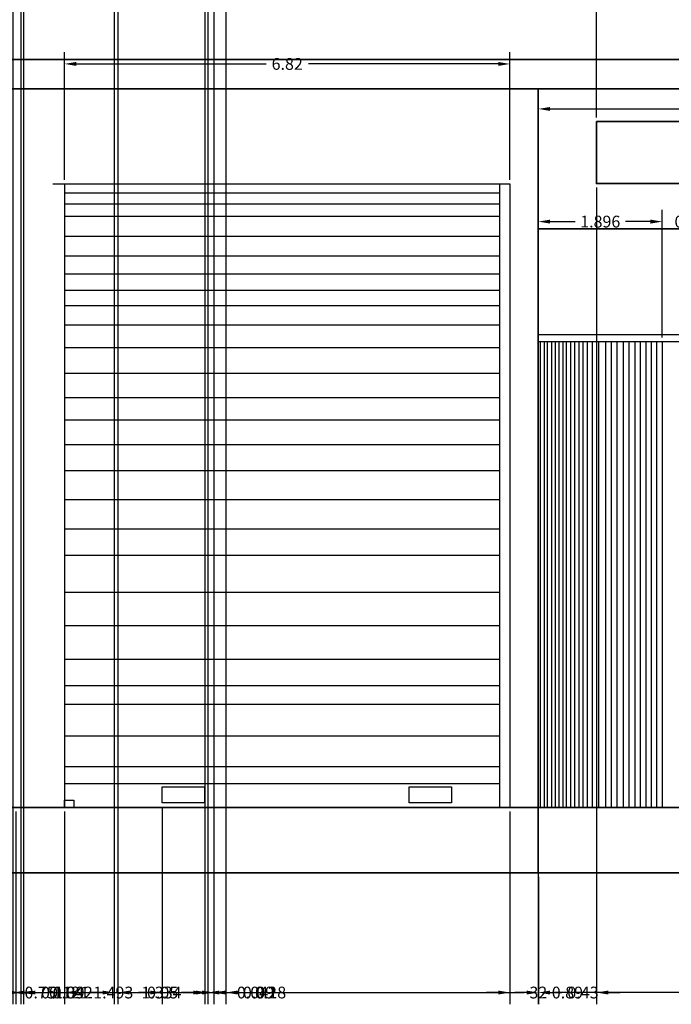
# Model space of a CAD drawing. Units: millimetres. Extents: x 2473 to 2512.3, y 2191.3 to 2230.4.
# Tile 2 of 8: x 2483.7 to 2493.7, y 2191.3 to 2206.4. Entities that reach past the tile are written whole.
import ezdxf

# ---------------------------------------------------------------- set-up
doc = ezdxf.new("R2010")
doc.units = ezdxf.units.MM
for name, color, linetype, lineweight in [('A-ANNO-DIMS', 2, 'Continuous', 18), ('A-DOOR', 4, 'Continuous', 25), ('A-ELEV', 7, 'Continuous', 35)]:
    doc.layers.add(name, color=color, linetype=linetype, lineweight=lineweight)
doc.styles.get("Standard").update_dxf_attribs({"font": 'arial.ttf'})
doc.dimstyles.get("Standard").update_dxf_attribs({"dimtxt": 0.18, "dimasz": 0.18, "dimexe": 0.18, "dimexo": 0.0625, "dimgap": 0.09, "dimtad": 0, "dimtih": 1, "dimtoh": 1, "dimdec": 4, "dimzin": 0, "dimdsep": 46, "dimtxsty": 'Standard', "dimcen": 0.09, "dimadec": 0, "dimazin": 0, "dimtfac": 1, "dimtdec": 4, "dimtofl": 0, "dimtmove": 0, "dimatfit": 3, "dimfxl": 1, "dimtolj": 1, "dimtzin": 0, "dimarcsym": 0})

# ---------------------------------------------------------------- blocks, each defined once
blk = doc.blocks.new('*D7')
at = {"layer": 'A-ANNO-DIMS', "color": 0, "lineweight": -2, "transparency": 16777216}
for p, q in [((2475.623, 2193.292), (2475.623, 2191.34)), ((2507.623, 2193.292), (2507.623, 2191.34)), ((2475.803, 2191.52), (2491.405, 2191.52)), ((2507.443, 2191.52), (2491.841, 2191.52))]:
    blk.add_line(p, q, dxfattribs=at)
at = {"layer": 'A-ANNO-DIMS', "color": 0, "transparency": 16777216}
for points in [[(2475.803, 2191.55), (2475.803, 2191.49), (2475.623, 2191.52)], [(2507.443, 2191.55), (2507.443, 2191.49), (2507.623, 2191.52)]]:
    blk.add_solid(points, dxfattribs=at)
at = {"layer": 'Defpoints', "color": 0, "transparency": 16777216}
for p in [(2475.623, 2193.355), (2507.623, 2193.355), (2507.623, 2191.52)]:
    blk.add_point(p, dxfattribs=at)
at = {"layer": 'A-ANNO-DIMS', "color": 0, "transparency": 16777216, "insert": (2491.623, 2191.52), "char_height": 0.18, "attachment_point": 5}
blk.add_mtext('\\A1;32', dxfattribs=at)
blk = doc.blocks.new('*D15')
at = {"layer": 'A-ANNO-DIMS', "color": 0, "lineweight": -2, "transparency": 16777216}
for p, q in [((2484.37, 2203.965), (2484.37, 2205.918)), ((2491.189, 2203.965), (2491.189, 2205.918)), ((2484.55, 2205.738), (2487.456, 2205.738)), ((2491.009, 2205.738), (2488.103, 2205.738))]:
    blk.add_line(p, q, dxfattribs=at)
at = {"layer": 'A-ANNO-DIMS', "color": 0, "transparency": 16777216}
for points in [[(2484.55, 2205.768), (2484.55, 2205.708), (2484.37, 2205.738)], [(2491.009, 2205.768), (2491.009, 2205.708), (2491.189, 2205.738)]]:
    blk.add_solid(points, dxfattribs=at)
at = {"layer": 'Defpoints', "color": 0, "transparency": 16777216}
for p in [(2491.189, 2205.738), (2484.37, 2203.903), (2491.189, 2203.903)]:
    blk.add_point(p, dxfattribs=at)
at = {"layer": 'A-ANNO-DIMS', "color": 0, "transparency": 16777216, "insert": (2487.779, 2205.738), "char_height": 0.18, "attachment_point": 5}
blk.add_mtext('\\A1;6.82', dxfattribs=at)
blk = doc.blocks.new('*D16')
at = {"layer": 'A-ANNO-DIMS', "color": 0, "lineweight": -2, "transparency": 16777216}
for p, q in [((2491.623, 2203.276), (2491.623, 2205.229)), ((2500.567, 2203.276), (2500.567, 2205.229)), ((2491.803, 2205.049), (2495.701, 2205.049)), ((2500.387, 2205.049), (2496.488, 2205.049))]:
    blk.add_line(p, q, dxfattribs=at)
at = {"layer": 'A-ANNO-DIMS', "color": 0, "transparency": 16777216}
for points in [[(2491.803, 2205.079), (2491.803, 2205.019), (2491.623, 2205.049)], [(2500.387, 2205.079), (2500.387, 2205.019), (2500.567, 2205.049)]]:
    blk.add_solid(points, dxfattribs=at)
at = {"layer": 'Defpoints', "color": 0, "transparency": 16777216}
for p in [(2500.567, 2205.049), (2491.623, 2203.214), (2500.567, 2203.214)]:
    blk.add_point(p, dxfattribs=at)
at = {"layer": 'A-ANNO-DIMS', "color": 0, "transparency": 16777216, "insert": (2496.095, 2205.049), "char_height": 0.18, "attachment_point": 5}
blk.add_mtext('\\A1;8.944', dxfattribs=at)
blk = doc.blocks.new('*D24')
at = {"layer": 'A-ANNO-DIMS', "color": 0, "lineweight": -2, "transparency": 16777216}
for p, q in [((2483.623, 2194.292), (2483.623, 2191.34)), ((2484.37, 2194.292), (2484.37, 2191.34)), ((2483.443, 2191.52), (2483.263, 2191.52)), ((2484.55, 2191.52), (2484.73, 2191.52))]:
    blk.add_line(p, q, dxfattribs=at)
at = {"layer": 'A-ANNO-DIMS', "color": 0, "transparency": 16777216}
for points in [[(2483.443, 2191.55), (2483.443, 2191.49), (2483.623, 2191.52)], [(2484.55, 2191.55), (2484.55, 2191.49), (2484.37, 2191.52)]]:
    blk.add_solid(points, dxfattribs=at)
at = {"layer": 'Defpoints', "color": 0, "transparency": 16777216}
for p in [(2483.623, 2194.355), (2484.37, 2194.355), (2484.37, 2191.52)]:
    blk.add_point(p, dxfattribs=at)
at = {"layer": 'A-ANNO-DIMS', "color": 0, "transparency": 16777216, "insert": (2483.996, 2191.52), "char_height": 0.18, "attachment_point": 5}
blk.add_mtext('\\A1;0.75', dxfattribs=at)
blk = doc.blocks.new('*D25')
at = {"layer": 'A-ANNO-DIMS', "color": 0, "lineweight": -2, "transparency": 16777216}
for p, q in [((2491.189, 2194.292), (2491.189, 2191.34)), ((2491.623, 2193.292), (2491.623, 2191.34)), ((2491.009, 2191.52), (2490.829, 2191.52)), ((2491.803, 2191.52), (2491.983, 2191.52))]:
    blk.add_line(p, q, dxfattribs=at)
at = {"layer": 'A-ANNO-DIMS', "color": 0, "transparency": 16777216}
for points in [[(2491.009, 2191.55), (2491.009, 2191.49), (2491.189, 2191.52)], [(2491.803, 2191.55), (2491.803, 2191.49), (2491.623, 2191.52)]]:
    blk.add_solid(points, dxfattribs=at)
at = {"layer": 'Defpoints', "color": 0, "transparency": 16777216}
for p in [(2491.189, 2194.355), (2491.623, 2193.355), (2491.623, 2191.52)]:
    blk.add_point(p, dxfattribs=at)
at = {"layer": 'A-ANNO-DIMS', "color": 0, "transparency": 16777216, "insert": (2492.307, 2191.52), "char_height": 0.18, "attachment_point": 5}
blk.add_mtext('\\A1;0.43', dxfattribs=at)
blk = doc.blocks.new('*D32')
at = {"layer": 'A-ANNO-DIMS', "color": 0, "lineweight": -2, "transparency": 16777216}
for p, q in [((2491.623, 2201.551), (2491.623, 2203.504)), ((2493.519, 2201.551), (2493.519, 2203.504)), ((2491.803, 2203.324), (2492.186, 2203.324)), ((2493.339, 2203.324), (2492.956, 2203.324))]:
    blk.add_line(p, q, dxfattribs=at)
at = {"layer": 'A-ANNO-DIMS', "color": 0, "transparency": 16777216}
for points in [[(2491.803, 2203.354), (2491.803, 2203.294), (2491.623, 2203.324)], [(2493.339, 2203.354), (2493.339, 2203.294), (2493.519, 2203.324)]]:
    blk.add_solid(points, dxfattribs=at)
at = {"layer": 'Defpoints', "color": 0, "transparency": 16777216}
for p in [(2493.519, 2203.324), (2491.623, 2201.489), (2493.519, 2201.489)]:
    blk.add_point(p, dxfattribs=at)
at = {"layer": 'A-ANNO-DIMS', "color": 0, "transparency": 16777216, "insert": (2492.571, 2203.324), "char_height": 0.18, "attachment_point": 5}
blk.add_mtext('\\A1;1.896', dxfattribs=at)
blk = doc.blocks.new('*D33')
at = {"layer": 'A-ANNO-DIMS', "color": 0, "lineweight": -2, "transparency": 16777216}
for p, q in [((2493.518828, 2201.551016), (2493.518828, 2203.503516)), ((2494.509822, 2201.551016), (2494.509822, 2203.503516)), ((2493.338828, 2203.323516), (2493.158828, 2203.323516)), ((2494.689822, 2203.323516), (2494.869822, 2203.323516))]:
    blk.add_line(p, q, dxfattribs=at)
at = {"layer": 'A-ANNO-DIMS', "color": 0, "transparency": 16777216}
for points in [[(2493.338828, 2203.353516), (2493.338828, 2203.293516), (2493.518828, 2203.323516)], [(2494.689822, 2203.353516), (2494.689822, 2203.293516), (2494.509822, 2203.323516)]]:
    blk.add_solid(points, dxfattribs=at)
at = {"layer": 'Defpoints', "color": 0, "transparency": 16777216}
for p in [(2494.509822, 2203.323516), (2493.518828, 2201.488516), (2494.509822, 2201.488516)]:
    blk.add_point(p, dxfattribs=at)
at = {"layer": 'A-ANNO-DIMS', "color": 0, "transparency": 16777216, "insert": (2494.014325, 2203.323516), "char_height": 0.18, "attachment_point": 5}
blk.add_mtext('\\A1;0.991', dxfattribs=at)
blk = doc.blocks.new('*D43')
at = {"layer": 'A-ANNO-DIMS', "color": 0, "lineweight": -2, "transparency": 16777216}
for p, q in [((2492.513324, 2203.844524), (2492.513324, 2191.339888)), ((2491.622904, 2203.151426), (2491.622904, 2191.339888)), ((2491.442904, 2191.519888), (2491.262904, 2191.519888)), ((2492.693324, 2191.519888), (2492.873324, 2191.519888))]:
    blk.add_line(p, q, dxfattribs=at)
at = {"layer": 'A-ANNO-DIMS', "color": 0, "transparency": 16777216}
for points in [[(2491.442904, 2191.549888), (2491.442904, 2191.489888), (2491.622904, 2191.519888)], [(2492.693324, 2191.549888), (2492.693324, 2191.489888), (2492.513324, 2191.519888)]]:
    blk.add_solid(points, dxfattribs=at)
at = {"layer": 'Defpoints', "color": 0, "transparency": 16777216}
for p in [(2492.513324, 2203.907024), (2491.622904, 2203.213926), (2492.513324, 2191.519888)]:
    blk.add_point(p, dxfattribs=at)
at = {"layer": 'A-ANNO-DIMS', "color": 0, "transparency": 16777216, "insert": (2492.068114, 2191.519888), "char_height": 0.18, "attachment_point": 5}
blk.add_mtext('\\A1;0.89', dxfattribs=at)
blk = doc.blocks.new('*D44')
at = {"layer": 'A-ANNO-DIMS', "color": 0, "lineweight": -2, "transparency": 16777216}
for p, q in [((2492.513, 2204.92), (2492.513, 2206.873)), ((2499.711, 2204.92), (2499.711, 2206.873)), ((2492.693, 2206.693), (2495.719, 2206.693)), ((2499.531, 2206.693), (2496.505, 2206.693))]:
    blk.add_line(p, q, dxfattribs=at)
at = {"layer": 'A-ANNO-DIMS', "color": 0, "transparency": 16777216}
for points in [[(2492.693, 2206.723), (2492.693, 2206.663), (2492.513, 2206.693)], [(2499.531, 2206.723), (2499.531, 2206.663), (2499.711, 2206.693)]]:
    blk.add_solid(points, dxfattribs=at)
at = {"layer": 'Defpoints', "color": 0, "transparency": 16777216}
for p in [(2499.711, 2206.693), (2492.513, 2204.858), (2499.711, 2204.858)]:
    blk.add_point(p, dxfattribs=at)
at = {"layer": 'A-ANNO-DIMS', "color": 0, "transparency": 16777216, "insert": (2496.112, 2206.693), "char_height": 0.18, "attachment_point": 5}
blk.add_mtext('\\A1;7.197', dxfattribs=at)
blk = doc.blocks.new('*D97')
at = {"layer": 'A-ANNO-DIMS', "color": 0, "lineweight": -2, "transparency": 16777216}
for p, q in [((2484.37, 2194.292), (2484.37, 2191.34)), ((2485.863, 2194.362), (2485.863, 2191.34)), ((2484.55, 2191.52), (2484.731, 2191.52)), ((2485.683, 2191.52), (2485.502, 2191.52))]:
    blk.add_line(p, q, dxfattribs=at)
at = {"layer": 'A-ANNO-DIMS', "color": 0, "transparency": 16777216}
for points in [[(2484.55, 2191.55), (2484.55, 2191.49), (2484.37, 2191.52)], [(2485.683, 2191.55), (2485.683, 2191.49), (2485.863, 2191.52)]]:
    blk.add_solid(points, dxfattribs=at)
at = {"layer": 'Defpoints', "color": 0, "transparency": 16777216}
for p in [(2485.863, 2194.424), (2484.37, 2194.355), (2485.863, 2191.52)]:
    blk.add_point(p, dxfattribs=at)
at = {"layer": 'A-ANNO-DIMS', "color": 0, "transparency": 16777216, "insert": (2485.116, 2191.52), "char_height": 0.18, "attachment_point": 5}
blk.add_mtext('\\A1;1.493', dxfattribs=at)
blk = doc.blocks.new('*D102')
at = {"layer": 'A-ANNO-DIMS', "color": 0, "lineweight": -2, "transparency": 16777216}
for p, q in [((2483.468, 2209.664), (2483.468, 2191.34)), ((2483.581, 2209.664), (2483.581, 2191.34)), ((2483.288, 2191.52), (2483.108, 2191.52)), ((2483.761, 2191.52), (2483.941, 2191.52))]:
    blk.add_line(p, q, dxfattribs=at)
at = {"layer": 'A-ANNO-DIMS', "color": 0, "transparency": 16777216}
for points in [[(2483.288, 2191.55), (2483.288, 2191.49), (2483.468, 2191.52)], [(2483.761, 2191.55), (2483.761, 2191.49), (2483.581, 2191.52)]]:
    blk.add_solid(points, dxfattribs=at)
at = {"layer": 'Defpoints', "color": 0, "transparency": 16777216}
for p in [(2483.468, 2209.727), (2483.581, 2209.727), (2483.581, 2191.52)]:
    blk.add_point(p, dxfattribs=at)
at = {"layer": 'A-ANNO-DIMS', "color": 0, "transparency": 16777216, "insert": (2484.248, 2191.52), "char_height": 0.18, "attachment_point": 5}
blk.add_mtext('\\A1;0.11', dxfattribs=at)
blk = doc.blocks.new('*D103')
at = {"layer": 'A-ANNO-DIMS', "color": 0, "lineweight": -2, "transparency": 16777216}
for p, q in [((2483.581, 2209.664), (2483.581, 2191.34)), ((2483.702, 2209.684), (2483.702, 2191.34)), ((2483.401, 2191.52), (2483.221, 2191.52)), ((2483.882, 2191.52), (2484.062, 2191.52))]:
    blk.add_line(p, q, dxfattribs=at)
at = {"layer": 'A-ANNO-DIMS', "color": 0, "transparency": 16777216}
for points in [[(2483.401, 2191.55), (2483.401, 2191.49), (2483.581, 2191.52)], [(2483.882, 2191.55), (2483.882, 2191.49), (2483.702, 2191.52)]]:
    blk.add_solid(points, dxfattribs=at)
at = {"layer": 'Defpoints', "color": 0, "transparency": 16777216}
for p in [(2483.581, 2209.727), (2483.702, 2209.747), (2483.702, 2191.52)]:
    blk.add_point(p, dxfattribs=at)
at = {"layer": 'A-ANNO-DIMS', "color": 0, "transparency": 16777216, "insert": (2484.439, 2191.52), "char_height": 0.18, "attachment_point": 5}
blk.add_mtext('\\A1;0.121', dxfattribs=at)
blk = doc.blocks.new('*D104')
at = {"layer": 'A-ANNO-DIMS', "color": 0, "lineweight": -2, "transparency": 16777216}
for p, q in [((2483.702, 2209.684), (2483.702, 2191.34)), ((2483.744, 2209.684), (2483.744, 2191.34)), ((2483.522, 2191.52), (2483.342, 2191.52)), ((2483.924, 2191.52), (2484.104, 2191.52))]:
    blk.add_line(p, q, dxfattribs=at)
at = {"layer": 'A-ANNO-DIMS', "color": 0, "transparency": 16777216}
for points in [[(2483.522, 2191.55), (2483.522, 2191.49), (2483.702, 2191.52)], [(2483.924, 2191.55), (2483.924, 2191.49), (2483.744, 2191.52)]]:
    blk.add_solid(points, dxfattribs=at)
at = {"layer": 'Defpoints', "color": 0, "transparency": 16777216}
for p in [(2483.702, 2209.747), (2483.744, 2209.747), (2483.744, 2191.52)]:
    blk.add_point(p, dxfattribs=at)
at = {"layer": 'A-ANNO-DIMS', "color": 0, "transparency": 16777216, "insert": (2484.497, 2191.52), "char_height": 0.18, "attachment_point": 5}
blk.add_mtext('\\A1;0.042', dxfattribs=at)
blk = doc.blocks.new('*D105')
at = {"layer": 'A-ANNO-DIMS', "color": 0, "lineweight": -2, "transparency": 16777216}
for p, q in [((2483.744, 2209.684), (2483.744, 2191.34)), ((2485.132, 2209.684), (2485.132, 2191.34)), ((2483.924, 2191.52), (2484.123, 2191.52)), ((2484.952, 2191.52), (2484.754, 2191.52))]:
    blk.add_line(p, q, dxfattribs=at)
at = {"layer": 'A-ANNO-DIMS', "color": 0, "transparency": 16777216}
for points in [[(2483.924, 2191.55), (2483.924, 2191.49), (2483.744, 2191.52)], [(2484.952, 2191.55), (2484.952, 2191.49), (2485.132, 2191.52)]]:
    blk.add_solid(points, dxfattribs=at)
at = {"layer": 'Defpoints', "color": 0, "transparency": 16777216}
for p in [(2483.744, 2209.747), (2485.132, 2209.747), (2485.132, 2191.52)]:
    blk.add_point(p, dxfattribs=at)
at = {"layer": 'A-ANNO-DIMS', "color": 0, "transparency": 16777216, "insert": (2484.438, 2191.52), "char_height": 0.18, "attachment_point": 5}
blk.add_mtext('\\A1;1.39', dxfattribs=at)
blk = doc.blocks.new('*D106')
at = {"layer": 'A-ANNO-DIMS', "color": 0, "lineweight": -2, "transparency": 16777216}
for p, q in [((2485.132, 2209.684), (2485.132, 2191.34)), ((2485.187, 2209.68), (2485.187, 2191.34)), ((2484.952, 2191.52), (2484.772, 2191.52)), ((2485.367, 2191.52), (2485.547, 2191.52))]:
    blk.add_line(p, q, dxfattribs=at)
at = {"layer": 'A-ANNO-DIMS', "color": 0, "transparency": 16777216}
for points in [[(2484.952, 2191.55), (2484.952, 2191.49), (2485.132, 2191.52)], [(2485.367, 2191.55), (2485.367, 2191.49), (2485.187, 2191.52)]]:
    blk.add_solid(points, dxfattribs=at)
at = {"layer": 'Defpoints', "color": 0, "transparency": 16777216}
for p in [(2485.132, 2209.747), (2485.187, 2209.743), (2485.187, 2191.52)]:
    blk.add_point(p, dxfattribs=at)
at = {"layer": 'A-ANNO-DIMS', "color": 0, "transparency": 16777216, "insert": (2485.871, 2191.52), "char_height": 0.18, "attachment_point": 5}
blk.add_mtext('\\A1;0.05', dxfattribs=at)
blk = doc.blocks.new('*D107')
at = {"layer": 'A-ANNO-DIMS', "color": 0, "lineweight": -2, "transparency": 16777216}
for p, q in [((2485.187, 2209.68), (2485.187, 2191.34)), ((2486.52, 2209.684), (2486.52, 2191.34)), ((2485.367, 2191.52), (2485.469, 2191.52)), ((2486.34, 2191.52), (2486.238, 2191.52))]:
    blk.add_line(p, q, dxfattribs=at)
at = {"layer": 'A-ANNO-DIMS', "color": 0, "transparency": 16777216}
for points in [[(2485.367, 2191.55), (2485.367, 2191.49), (2485.187, 2191.52)], [(2486.34, 2191.55), (2486.34, 2191.49), (2486.52, 2191.52)]]:
    blk.add_solid(points, dxfattribs=at)
at = {"layer": 'Defpoints', "color": 0, "transparency": 16777216}
for p in [(2485.187, 2209.743), (2486.52, 2209.747), (2486.52, 2191.52)]:
    blk.add_point(p, dxfattribs=at)
at = {"layer": 'A-ANNO-DIMS', "color": 0, "transparency": 16777216, "insert": (2485.854, 2191.52), "char_height": 0.18, "attachment_point": 5}
blk.add_mtext('\\A1;1.334', dxfattribs=at)
blk = doc.blocks.new('*D108')
at = {"layer": 'A-ANNO-DIMS', "color": 0, "lineweight": -2, "transparency": 16777216}
for p, q in [((2486.52, 2209.684), (2486.52, 2191.34)), ((2486.562, 2209.684), (2486.562, 2191.34)), ((2486.34, 2191.52), (2486.16, 2191.52)), ((2486.742, 2191.52), (2486.922, 2191.52))]:
    blk.add_line(p, q, dxfattribs=at)
at = {"layer": 'A-ANNO-DIMS', "color": 0, "transparency": 16777216}
for points in [[(2486.34, 2191.55), (2486.34, 2191.49), (2486.52, 2191.52)], [(2486.742, 2191.55), (2486.742, 2191.49), (2486.562, 2191.52)]]:
    blk.add_solid(points, dxfattribs=at)
at = {"layer": 'Defpoints', "color": 0, "transparency": 16777216}
for p in [(2486.52, 2209.747), (2486.562, 2209.747), (2486.562, 2191.52)]:
    blk.add_point(p, dxfattribs=at)
at = {"layer": 'A-ANNO-DIMS', "color": 0, "transparency": 16777216, "insert": (2487.315, 2191.52), "char_height": 0.18, "attachment_point": 5}
blk.add_mtext('\\A1;0.042', dxfattribs=at)
blk = doc.blocks.new('*D109')
at = {"layer": 'A-ANNO-DIMS', "color": 0, "lineweight": -2, "transparency": 16777216}
for p, q in [((2486.562, 2209.684), (2486.562, 2191.34)), ((2486.655, 2209.664), (2486.655, 2191.34)), ((2486.382, 2191.52), (2486.202, 2191.52)), ((2486.835, 2191.52), (2487.015, 2191.52))]:
    blk.add_line(p, q, dxfattribs=at)
at = {"layer": 'A-ANNO-DIMS', "color": 0, "transparency": 16777216}
for points in [[(2486.382, 2191.55), (2486.382, 2191.49), (2486.562, 2191.52)], [(2486.835, 2191.55), (2486.835, 2191.49), (2486.655, 2191.52)]]:
    blk.add_solid(points, dxfattribs=at)
at = {"layer": 'Defpoints', "color": 0, "transparency": 16777216}
for p in [(2486.562, 2209.747), (2486.655, 2209.727), (2486.655, 2191.52)]:
    blk.add_point(p, dxfattribs=at)
at = {"layer": 'A-ANNO-DIMS', "color": 0, "transparency": 16777216, "insert": (2487.339, 2191.52), "char_height": 0.18, "attachment_point": 5}
blk.add_mtext('\\A1;0.09', dxfattribs=at)
blk = doc.blocks.new('*D110')
at = {"layer": 'A-ANNO-DIMS', "color": 0, "lineweight": -2, "transparency": 16777216}
for p, q in [((2486.655, 2209.664), (2486.655, 2191.34)), ((2486.84, 2209.664), (2486.84, 2191.34)), ((2486.475, 2191.52), (2486.295, 2191.52)), ((2487.02, 2191.52), (2487.2, 2191.52))]:
    blk.add_line(p, q, dxfattribs=at)
at = {"layer": 'A-ANNO-DIMS', "color": 0, "transparency": 16777216}
for points in [[(2486.475, 2191.55), (2486.475, 2191.49), (2486.655, 2191.52)], [(2487.02, 2191.55), (2487.02, 2191.49), (2486.84, 2191.52)]]:
    blk.add_solid(points, dxfattribs=at)
at = {"layer": 'Defpoints', "color": 0, "transparency": 16777216}
for p in [(2486.655, 2209.727), (2486.84, 2209.727), (2486.84, 2191.52)]:
    blk.add_point(p, dxfattribs=at)
at = {"layer": 'A-ANNO-DIMS', "color": 0, "transparency": 16777216, "insert": (2487.524, 2191.52), "char_height": 0.18, "attachment_point": 5}
blk.add_mtext('\\A1;0.18', dxfattribs=at)

msp = doc.modelspace()

# ---------------------------------------------------------------- linework, layer by layer
at = {"layer": 'A-DOOR'}
for p, q in [((2484.1891, 2203.9027), (2491.1891, 2203.9027)), ((2484.3698, 2203.9027), (2484.3698, 2194.3549)), ((2491.0302, 2203.9027), (2491.0302, 2194.3549)), ((2491.1891, 2203.9027), (2491.1891, 2194.3549)), ((2484.3698, 2203.7647), (2491.0302, 2203.7647)), ((2484.3698, 2203.5963), (2491.0302, 2203.5963)), ((2484.3698, 2203.4067), (2491.0302, 2203.4067)), ((2484.3698, 2203.1), (2491.0302, 2203.1)), ((2484.3698, 2202.7988), (2491.0302, 2202.7988)), ((2484.3698, 2202.5255), (2491.0302, 2202.5255)), ((2484.3698, 2202.2745), (2491.0302, 2202.2745)), ((2484.3698, 2202.0402), (2491.0302, 2202.0402)), ((2484.3698, 2201.7408), (2491.0302, 2201.7408)), ((2491.6229, 2201.5952), (2500.5668, 2201.5952)), ((2491.6229, 2201.4885), (2500.5668, 2201.4885)), ((2491.6525, 2201.4885), (2491.6525, 2194.3549)), ((2491.7101, 2201.4885), (2491.7101, 2194.3549)), ((2491.7603, 2201.4885), (2491.7603, 2194.3549)), ((2491.8259, 2201.4885), (2491.8259, 2194.3549)), ((2491.8794, 2201.4885), (2491.8794, 2194.3549)), ((2491.9381, 2201.4885), (2491.9381, 2194.3549)), ((2491.9967, 2201.4885), (2491.9967, 2194.3549)), ((2492.0502, 2201.4885), (2492.0502, 2194.3549)), ((2492.1141, 2201.4885), (2492.1141, 2194.3549)), ((2492.178, 2201.4885), (2492.178, 2194.3549)), ((2492.2435, 2201.4885), (2492.2435, 2194.3549)), ((2492.3057, 2201.4885), (2492.3057, 2194.3549)), ((2492.369, 2201.4885), (2492.369, 2194.3549)), ((2492.4481, 2201.4885), (2492.4481, 2194.3549)), ((2492.5436, 2201.4885), (2492.5436, 2194.3549)), ((2492.6499, 2201.4885), (2492.6499, 2194.3549)), ((2492.74, 2201.4885), (2492.74, 2194.3549)), ((2492.8272, 2201.4885), (2492.8272, 2194.3549)), ((2492.9227, 2201.4885), (2492.9227, 2194.3549)), ((2493.01, 2201.4885), (2493.01, 2194.3549)), ((2493.1, 2201.4885), (2493.1, 2194.3549)), ((2493.1818, 2201.4885), (2493.1818, 2194.3549)), ((2493.2691, 2201.4885), (2493.2691, 2194.3549)), ((2493.3509, 2201.4885), (2493.3509, 2194.3549)), ((2493.4328, 2201.4885), (2493.4328, 2194.3549)), ((2493.5188, 2201.4885), (2493.5188, 2194.3549)), ((2484.3698, 2201.3981), (2491.0302, 2201.3981)), ((2484.3698, 2201.0013), (2491.0302, 2201.0013)), ((2484.3698, 2200.6315), (2491.0302, 2200.6315)), ((2484.3698, 2200.2888), (2491.0302, 2200.2888)), ((2484.3698, 2199.91), (2491.0302, 2199.91)), ((2484.3698, 2199.5132), (2491.0302, 2199.5132)), ((2484.3698, 2199.0712), (2491.0302, 2199.0712)), ((2484.3698, 2198.621), (2491.0302, 2198.621)), ((2484.3698, 2198.218), (2491.0302, 2198.218)), ((2484.3698, 2197.6503), (2491.0302, 2197.6503)), ((2484.3698, 2197.1375), (2491.0302, 2197.1375)), ((2484.3698, 2196.6247), (2491.0302, 2196.6247)), ((2484.3698, 2196.2209), (2491.0302, 2196.2209)), ((2484.3698, 2195.9338), (2491.0302, 2195.9338)), ((2484.3698, 2195.4522), (2491.0302, 2195.4522)), ((2484.3698, 2194.9798), (2491.0302, 2194.9798)), ((2484.3698, 2194.7229), (2491.0302, 2194.7229))]:
    msp.add_line(p, q, dxfattribs=at)
for points in [[(2485.8628, 2194.6682), (2486.5134, 2194.6682), (2486.5134, 2194.4242), (2485.8628, 2194.4242)], [(2489.6445, 2194.6682), (2490.2951, 2194.6682), (2490.2951, 2194.4242), (2489.6445, 2194.4242)], [(2484.3698, 2194.4642), (2484.5113, 2194.4642), (2484.5113, 2194.3549), (2484.3698, 2194.3549)]]:
    msp.add_lwpolyline(points, close=True, dxfattribs=at)
at = {"layer": 'A-ELEV'}
for p, q in [((2507.6229, 2205.8077), (2475.6229, 2205.8077)), ((2507.6229, 2205.3549), (2475.6229, 2205.3549)), ((2491.6229, 2193.3549), (2491.6229, 2205.3549)), ((2491.6229, 2203.2139), (2500.5668, 2203.2139)), ((2491.6229, 2194.3549), (2475.6229, 2194.3549)), ((2507.6229, 2194.3549), (2491.6229, 2194.3549)), ((2507.6229, 2193.3549), (2475.6229, 2193.3549))]:
    msp.add_line(p, q, dxfattribs=at)
msp.add_lwpolyline([(2492.5133, 2204.8576), (2499.7107, 2204.8576), (2499.7107, 2203.907), (2492.5133, 2203.907)], close=True, dxfattribs=at)

# ---------------------------------------------------------------- dimensions: what is measured, and where the dimension line sits
at = {"layer": 'A-ANNO-DIMS'}
for base, p1, p2, override, picture, middle in [((2483.5812, 2191.5199), (2483.4683, 2209.7269), (2483.5812, 2209.7269), {"dimdec": 2, "dimlfac": 1, "dimrnd": 0, "dimzin": 0, "dimdsep": 46, "dimlunit": 2}, '*D102', (2484.2476, 2191.5199)), ((2483.7022, 2191.5199), (2483.5812, 2209.7269), (2483.7022, 2209.7466), {"dimdec": 3, "dimlfac": 1, "dimrnd": 0, "dimzin": 0, "dimdsep": 46, "dimlunit": 2}, '*D103', (2484.4385, 2191.5199)), ((2483.7441, 2191.5199), (2483.7022, 2209.7466), (2483.7441, 2209.7466), {"dimdec": 3, "dimlfac": 1, "dimrnd": 0, "dimzin": 0, "dimdsep": 46, "dimlunit": 2}, '*D104', (2484.4969, 2191.5199)), ((2485.1323, 2191.5199), (2483.7441, 2209.7466), (2485.1323, 2209.7466), {"dimdec": 2, "dimlfac": 1, "dimrnd": 0, "dimzin": 0, "dimdsep": 46, "dimlunit": 2}, '*D105', (2484.4382, 2191.5199)), ((2485.1866, 2191.5199), (2485.1323, 2209.7466), (2485.1866, 2209.7428), {"dimdec": 2, "dimlfac": 1, "dimrnd": 0, "dimzin": 0, "dimdsep": 46, "dimlunit": 2}, '*D106', (2485.871, 2191.5199)), ((2486.5205, 2191.5199), (2485.1866, 2209.7428), (2486.5205, 2209.7466), {"dimdec": 3, "dimlfac": 1, "dimrnd": 0, "dimzin": 0, "dimdsep": 46, "dimlunit": 2}, '*D107', (2485.8535, 2191.5199)), ((2486.5624, 2191.5199), (2486.5205, 2209.7466), (2486.5624, 2209.7466), {"dimdec": 3, "dimlfac": 1, "dimrnd": 0, "dimzin": 0, "dimdsep": 46, "dimlunit": 2}, '*D108', (2487.3152, 2191.5199)), ((2486.655, 2191.5199), (2486.5624, 2209.7466), (2486.655, 2209.7269), {"dimdec": 2, "dimlfac": 1, "dimrnd": 0, "dimzin": 0, "dimdsep": 46, "dimlunit": 2}, '*D109', (2487.339, 2191.5199)), ((2486.8395, 2191.5199), (2486.655, 2209.7269), (2486.8395, 2209.7269), {"dimdec": 2, "dimlfac": 1, "dimrnd": 0, "dimzin": 0, "dimdsep": 46, "dimlunit": 2}, '*D110', (2487.5235, 2191.5199)), ((2499.7107, 2206.6926), (2492.5133, 2204.8576), (2499.7107, 2204.8576), {"dimdec": 3, "dimlfac": 1, "dimrnd": 0, "dimzin": 0, "dimdsep": 46, "dimlunit": 2}, '*D44', (2496.112, 2206.6926)), ((2491.1891, 2205.7377), (2484.3698, 2203.9027), (2491.1891, 2203.9027), {"dimdec": 2, "dimlfac": 1, "dimrnd": 0, "dimzin": 0, "dimdsep": 46, "dimlunit": 2}, '*D15', (2487.7795, 2205.7377)), ((2500.5668, 2205.0489), (2491.6229, 2203.2139), (2500.5668, 2203.2139), {"dimdec": 3, "dimlfac": 1, "dimrnd": 0, "dimzin": 0, "dimdsep": 46, "dimlunit": 2}, '*D16', (2496.0949, 2205.0489)), ((2492.5133, 2191.5199), (2491.6229, 2203.2139), (2492.5133, 2203.907), {"dimdec": 2, "dimlfac": 1, "dimrnd": 0, "dimzin": 0, "dimdsep": 46, "dimlunit": 2}, '*D43', (2492.0681, 2191.5199)), ((2493.5188, 2203.3235), (2491.6229, 2201.4885), (2493.5188, 2201.4885), {"dimdec": 3, "dimlfac": 1, "dimrnd": 0, "dimzin": 0, "dimdsep": 46, "dimlunit": 2}, '*D32', (2492.5709, 2203.3235)), ((2494.5098, 2203.3235), (2493.5188, 2201.4885), (2494.5098, 2201.4885), {"dimdec": 3, "dimlfac": 1, "dimrnd": 0, "dimzin": 0, "dimdsep": 46, "dimlunit": 2}, '*D33', (2494.0143, 2203.3235)), ((2485.8628, 2191.5199), (2484.3698, 2194.3549), (2485.8628, 2194.4242), {"dimdec": 3, "dimlfac": 1, "dimrnd": 0, "dimzin": 0, "dimdsep": 46, "dimlunit": 2}, '*D97', (2485.1163, 2191.5199)), ((2484.3698, 2191.5199), (2483.6229, 2194.3549), (2484.3698, 2194.3549), {"dimdec": 2, "dimlfac": 1, "dimrnd": 0, "dimzin": 0, "dimdsep": 46, "dimlunit": 2}, '*D24', (2483.9963, 2191.5199)), ((2491.6229, 2191.5199), (2491.1891, 2194.3549), (2491.6229, 2193.3549), {"dimdec": 2, "dimlfac": 1, "dimrnd": 0, "dimzin": 0, "dimdsep": 46, "dimlunit": 2}, '*D25', (2492.3067, 2191.5199)), ((2507.6229, 2191.5199), (2475.6229, 2193.3549), (2507.6229, 2193.3549), {"dimdec": 0, "dimlfac": 1, "dimrnd": 0, "dimzin": 0, "dimdsep": 46, "dimlunit": 2}, '*D7', (2491.6229, 2191.5199))]:
    dim = msp.add_linear_dim(base=base, p1=p1, p2=p2, dimstyle='Standard', override=override, dxfattribs=at)
    dim.commit()
    dim.dimension.update_dxf_attribs({"geometry": picture, "text_midpoint": middle})

doc.saveas('drawing.dxf')
